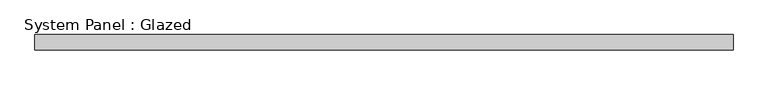
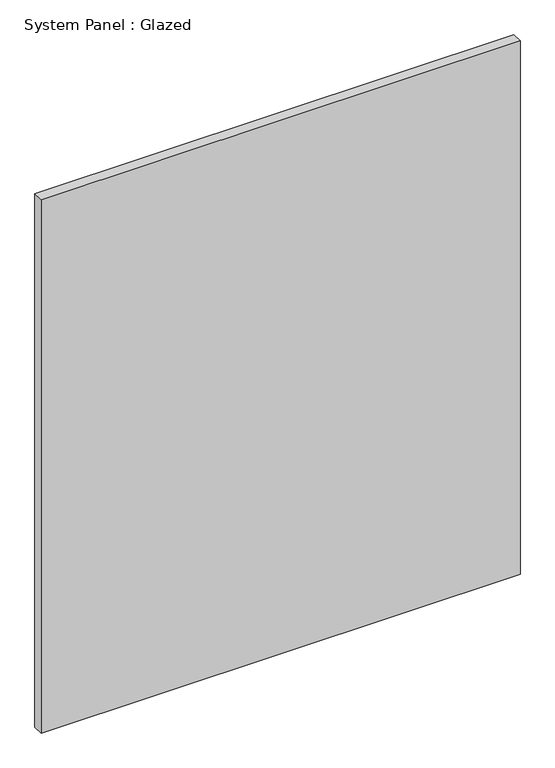
"""IFC4 building model written with IfcOpenShell, lengths in millimetres: plate geometry, System Panel : Glazed."""

from ifc_helpers import new_model, si_unit, origin, origin_with_axes, place, context, project, spatial, polyline, outline, extrude, source, transform, mapped, element, save


def system_panel_glazed_e1dbe616(model_context):
    return source(origin(), model_context, "Body", "SweptSolid", [
        extrude(outline(polyline([(565.15, 24.5), (-565.15, 24.5), (-565.15, 49.5), (565.15, 49.5), (565.15, 24.5)])), origin_with_axes(), (0.0, 0.0, 1.0), 1330.8429687),
    ])


if __name__ == "__main__":
    model = new_model("IFC4")
    model_context = context("Model", 3, world=origin())
    ifc_project = project(units=[si_unit("LENGTHUNIT", "METRE", prefix="MILLI")], contexts=[model_context])
    site = spatial("IfcSite", under=ifc_project)
    building = spatial("IfcBuilding", under=site)
    placement = place(None, origin())
    system_panel_glazed_shape = system_panel_glazed_e1dbe616(model_context)
    element("IfcPlate", 1, ObjectType="System Panel : Glazed", at=placement, inside=building, context=model_context, shape_type="MappedRepresentation", body=[
        mapped(system_panel_glazed_shape, transform((0.0, 0.0, 0.0), x_axis=(1.0, 0.0, 0.0), y_axis=(0.0, 1.0, 0.0), z_axis=(0.0, 0.0, 1.0))),
    ])
    save(model, "model.ifc")

# Revit data of these elements
# Type "System Panel : Glazed"
#   Keynote = "H11"
#   Construction Type Id = "GSP4R"
#   Analytic Construction = "1/8 in Pilkington single glazing"
#   Visual Light Transmittance = 0.9
#   Solar Heat Gain Coefficient = 0.86
#   Heat Transfer Coefficient (U) = 6.7069 W/(m²·K)
#   Define Thermal Properties by = 1
# Element 1 (IfcPlate, "System Panel : Glazed")
#   Materials on its faces: "Glass"
# Materials
#   "Glass": class "Glass", colour RGB 0 128 192, transparency 0.9, Description = "Soda Lime Glass", Cost = 0
